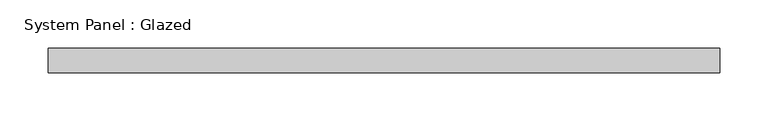
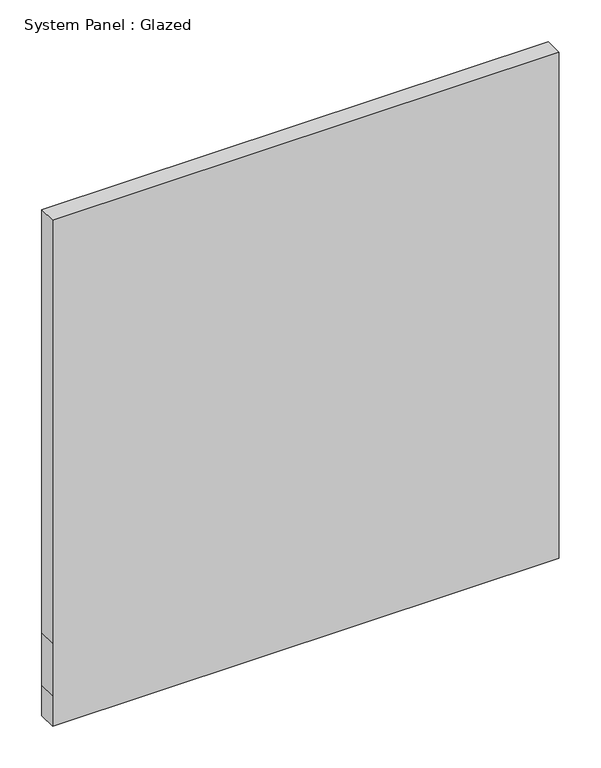
"""IFC4 building model written with IfcOpenShell, lengths in millimetres: plate geometry, System Panel : Glazed."""

from ifc_helpers import new_model, si_unit, frame, origin, place, context, project, spatial, polyline, outline, extrude, source, transform, mapped, element, save


def system_panel_glazed_1b56a55a(model_context):
    return source(origin(), model_context, "Body", "SweptSolid", [
        extrude(outline(polyline([(0.0, -349.25), (0.0, 349.25), (44.45, 349.25), (120.65, 349.25), (737.1888769, 349.25), (737.1888769, -349.25), (120.65, -349.25), (44.45, -349.25), (0.0, -349.25)])), frame((0.0, 19.05, 0.0), z_axis=(0.0, 1.0, 0.0), x_axis=(0.0, 0.0, 1.0)), (0.0, 0.0, 1.0), 25.4),
    ])


if __name__ == "__main__":
    model = new_model("IFC4")
    model_context = context("Model", 3, world=origin())
    ifc_project = project(units=[si_unit("LENGTHUNIT", "METRE", prefix="MILLI")], contexts=[model_context])
    site = spatial("IfcSite", under=ifc_project)
    building = spatial("IfcBuilding", under=site)
    placement = place(None, origin())
    system_panel_glazed_shape = system_panel_glazed_1b56a55a(model_context)
    element("IfcPlate", 1, ObjectType="System Panel : Glazed", at=placement, inside=building, context=model_context, shape_type="MappedRepresentation", body=[
        mapped(system_panel_glazed_shape, transform((0.0, 0.0, 0.0), x_axis=(1.0, 0.0, 0.0), y_axis=(0.0, 1.0, 0.0), z_axis=(0.0, 0.0, 1.0))),
    ])
    save(model, "model.ifc")

# Revit data of these elements
# Type "System Panel : Glazed"
#   Construction Type Id = "GSP4R"
#   Analytic Construction = "1/8 in Pilkington single glazing"
#   Visual Light Transmittance = 0.9
#   Solar Heat Gain Coefficient = 0.86
#   Heat Transfer Coefficient (U) = 1.18115 BTU/(h·ft²·°F)
#   Define Thermal Properties by = 1
# Element 1 (IfcPlate, "System Panel : Glazed")
#   Materials on its faces: "Glass"
# Materials
#   "Glass": class "Glass", colour RGB 0 128 192, transparency 0.75, Description = "Soda Lime Glass", Cost = 0
